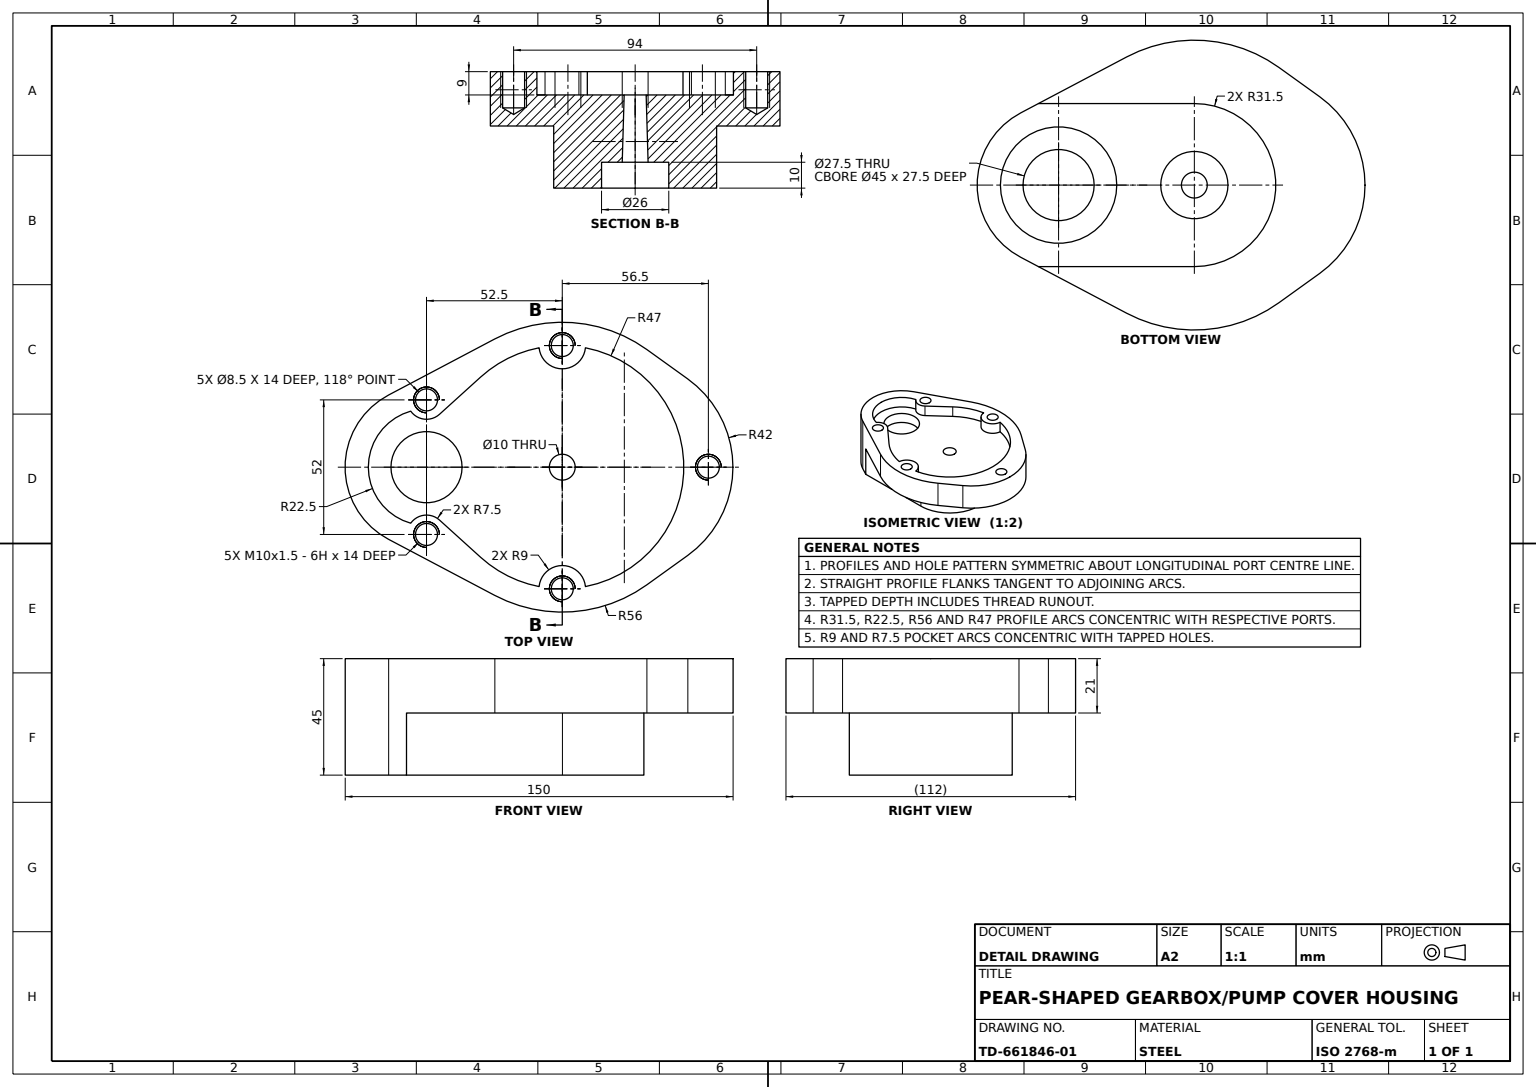
SolidWorks part; units mm, degrees
material "Plain Carbon Steel"
ref_plane "Front Plane" through (0, 0, 0) normal (0, 0, 1) x (1, 0, 0)
ref_plane "Top Plane" through (0, 0, 0) normal (0, 1, 0) x (1, 0, 0)
ref_plane "Right Plane" through (0, 0, 0) normal (1, 0, 0) x (0, 0, -1)
sketch "Flange Base Profile" plane through (0, 0, 0) normal (0, 1, 0) x (1, 0, 0)
  line L0 (-49.5283, 26.3667) -> (-27.8596, -14.7)
  line L1 (27.8596, -14.7) -> (49.5283, 26.3667)
  line L2 (0, 0) -> (0, 118.5) construction
  line L3 (-45.485, 85.1667) -> (-34.1138, 101)
  line L4 (45.485, 85.1667) -> (34.1138, 101)
  arc A0 (-27.8596, -14.7) -> (27.8596, -14.7) centre (0, 0) ccw
  arc A1 (49.5283, 26.3667) -> (45.485, 85.1667) centre (0, 52.5) ccw
  arc A2 (34.1138, 101) -> (-34.1138, 101) centre (0, 76.5) ccw
  arc A3 (-45.485, 85.1667) -> (-49.5283, 26.3667) centre (0, 52.5) ccw
  point P9 (0, -31.5)
  point P15 (0, 109)
  dimension "D1" = 31.5
  dimension "D2" = 56
  dimension "D4" = 42
  dimension "D3" = 52.5
  dimension "D5" = 150
  dimension "D6" = 56.5
extrude "Flange Base 21mm" add sketch "Flange Base Profile" along normal blind 21
sketch "Port Pocket Profile" plane through (0, 21, 0) normal (0, 1, 0) x (1, 0, 0)
  line L0 (0, 0) -> (0, -14.6458) construction
  line L1 (-21.5965, 6.3121) -> (-20.4378, 5.0311)
  line L2 (34.8564, 20.9717) -> (20.4378, 5.0311)
  line L3 (-34.8564, 20.9717) -> (-21.5965, 6.3121)
  arc A0 (-46.1383, 43.5413) -> (-34.8564, 20.9717) centre (0, 52.5) ccw
  arc A1 (49.5283, 26.3667) -> (45.485, 85.1667) centre (0, 52.5) ccw construction
  arc A2 (-46.1383, 43.5413) -> (-46.1383, 61.4587) centre (-47, 52.5) ccw
  arc A3 (-46.1383, 61.4587) -> (-46.1383, 43.5413) centre (-47, 52.5) ccw construction
  arc A4 (-46.1383, 61.4587) -> (-46.1383, 43.5413) centre (0, 52.5) ccw construction
  arc A5 (46.1383, 43.5413) -> (46.1383, 61.4587) centre (47, 52.5) cw
  arc A6 (46.1383, 43.5413) -> (46.1383, 61.4587) centre (0, 52.5) ccw construction
  arc A7 (46.1383, 61.4587) -> (-46.1383, 61.4587) centre (0, 52.5) ccw
  arc A8 (-21.5965, 6.3121) -> (-21.6538, 6.1124) centre (0, 0) ccw construction
  arc A9 (-20.1391, 10.0333) -> (20.1391, 10.0333) centre (0, 52.5) ccw construction
  arc A10 (34.8564, 20.9717) -> (46.1383, 43.5413) centre (0, 52.5) ccw
  arc A11 (20.1391, 10.0333) -> (-20.1391, 10.0333) centre (0, 0) ccw construction
  arc A12 (-21.6538, -6.1124) -> (-20.4378, 5.0311) centre (-26, 0) ccw
  arc A13 (21.6538, -6.1124) -> (20.4378, 5.0311) centre (26, 0) cw
  arc A14 (-20.1391, 10.0333) -> (-21.5965, 6.3121) centre (0, 0) ccw construction
  arc A15 (-34.8564, 20.9717) -> (-20.1391, 10.0333) centre (0, 52.5) ccw construction
  arc A16 (21.5965, 6.3121) -> (20.1391, 10.0333) centre (0, 0) ccw construction
  arc A17 (20.1391, 10.0333) -> (34.8564, 20.9717) centre (0, 52.5) ccw construction
  arc A18 (-21.6538, 6.1124) -> (-21.6538, -6.1124) centre (-26, 0) ccw construction
  arc A19 (-21.6538, 6.1124) -> (-21.6538, -6.1124) centre (0, 0) ccw construction
  arc A20 (-21.6538, -6.1124) -> (21.6538, -6.1124) centre (0, 0) ccw
  arc A21 (21.6538, -6.1124) -> (21.6538, 6.1124) centre (0, 0) ccw construction
  arc A22 (21.6538, 6.1124) -> (21.5965, 6.3121) centre (0, 0) ccw construction
  arc A23 (21.6538, 6.1124) -> (21.6538, -6.1124) centre (26, 0) cw construction
  arc A24 (-20.4378, 5.0311) -> (-21.6538, 6.1124) centre (-26, 0) ccw construction
  arc A25 (20.4378, 5.0311) -> (21.6538, 6.1124) centre (26, 0) cw construction
  dimension "D1" = 47
  dimension "D2" = 9
  dimension "D3" = 22.5
  dimension "D4" = 7.5
  dimension "D5" = 52
extrude "Port Pocket 9mm Deep" cut sketch "Port Pocket Profile" against normal blind 9
hole_wizard "Tapped Hole M10 Drill Ø8.5" positions "3DSketch2" profile "Sketch4" hole size "M10" standard "ISO"
sketch3d "3DSketch2"
  line L0 (-47, 12, -52.5) -> (-47, 21, -52.5) construction
  arc A0 (-46.1383, 21, -61.4587) -> (-46.1383, 21, -43.5413) centre (-47, 21, -52.5) ccw construction
  arc A1 (46.1383, 21, -43.5413) -> (46.1383, 21, -61.4587) centre (47, 21, -52.5) ccw construction
  arc A2 (21.6538, 21, 6.1124) -> (20.4378, 21, -5.0311) centre (26, 21, 0) ccw construction
  arc A3 (-20.4378, 21, -5.0311) -> (-21.6538, 21, 6.1124) centre (-26, 21, 0) ccw construction
  point P0 (0, 21, -109)
  point P5 (-47, 21, -52.5)
  point P9 (47, 21, -52.5)
  point P11 (-26, 21, 0)
  point P13 (26, 21, 0)
  point P18 (-47, 12, -52.5)
  point P22 (47, 12, -52.5)
  point P26 (26, 13.5, 0)
  point P30 (-26, 13.5, 0)
sketch "Sketch4" plane through (0, 21, -109) normal (1, 0, 0) x (0, 0, 1)
  line L0 (0, 0) -> (0, 16.5537)
  line L1 (0, 16.5537) -> (4.25, 14)
  line L2 (4.25, 14) -> (4.25, 0)
  line L5 (4.25, 0) -> (0, 0)
  line L10 (0, 16.5537) -> (-4.25, 14) construction
  line L11 (0, -6.35) -> (0, 107.95) construction
  dimension "Hole Dia." = 8.5
  dimension "Hole Depth" = 14
  dimension "Drill Angle" = 118
sketch "Port Boss Profile" plane through (0, 0, 0) normal (0, -1, 0) x (1, 0, 0)
  line L6 (0, 0) -> (0, -52.5) construction
  line L11 (31.5, 0) -> (31.5, -52.5)
  line L12 (-31.5, 0) -> (-31.5, -52.5)
  line L15 (-31.5, 0) -> (-31.5, 7.8008)
  line L17 (-49.5283, -26.3667) -> (-27.8596, 14.7) construction
  line L18 (-31.5, 7.8008) -> (-27.8596, 14.7)
  line L19 (31.5, 0) -> (31.5, 7.8008)
  line L20 (27.8596, 14.7) -> (49.5283, -26.3667) construction
  line L21 (27.8596, 14.7) -> (31.5, 7.8008)
  arc A3 (27.8596, 14.7) -> (-27.8596, 14.7) centre (0, 0) ccw
  arc A6 (-31.5, -52.5) -> (31.5, -52.5) centre (0, -52.5) ccw
  arc A7 (-27.8596, 14.7) -> (-31.5, 0) centre (0, 0) ccw construction
  arc A8 (31.5, 0) -> (27.8596, 14.7) centre (0, 0) ccw construction
  dimension "D1" = 52.5
  dimension "D2" = 31.5
extrude "Port Boss 24mm" add sketch "Port Boss Profile" along normal blind 24
hole_wizard "Main Port C-Bore Ø27.5" positions "3DSketch3" profile "Sketch7" legacy
sketch3d "3DSketch3"
  arc A0 (27.8596, -24, 14.7) -> (-27.8596, -24, 14.7) centre (0, -24, 0) ccw construction
  point P0 (0, 0, 0)
  point P3 (0, -24, 0)
  point P9 (0, -55.5, 0)
sketch "Sketch7" plane through (0, -24, 0) normal (1, 0, 0) x (0, 0, -1)
  line L0 (0, 0) -> (0, 99.6165)
  line L1 (0, 99.6165) -> (13.75, 99.6165)
  line L2 (13.75, 99.6165) -> (13.75, 27.5)
  line L3 (13.75, 27.5) -> (22.5, 27.5)
  line L4 (22.5, 27.5) -> (22.5, 0)
  line L5 (22.5, 0) -> (0, 0)
  line L6 (0, 110) -> (0, -10) construction
  dimension "Diameter" = 27.5
  dimension "Depth" = 100
  dimension "C-Bore Diameter" = 45
  dimension "C-Bore Depth" = 27.5
hole_wizard "Secondary Port C-Bore Ø10" positions "3DSketch4" profile "Sketch8" legacy
sketch3d "3DSketch4"
  arc A0 (-31.5, 0, -52.5) -> (31.5, 0, -52.5) centre (0, 0, -52.5) ccw construction
  point P0 (0, -24, -52.5)
  point P6 (0, -31.5, -52.5)
sketch "Sketch8" plane through (0, -24, -52.5) normal (1, 0, 0) x (0, 0, -1)
  line L0 (0, 0) -> (0, 99.6795)
  line L1 (0, 99.6795) -> (5, 99.6795)
  line L2 (5, 99.6795) -> (5, 10)
  line L3 (5, 10) -> (13, 10)
  line L4 (13, 10) -> (13, 0)
  line L5 (13, 0) -> (0, 0)
  line L6 (0, 110) -> (0, -10) construction
  dimension "Diameter" = 10
  dimension "Depth" = 100
  dimension "C-Bore Diameter" = 26
  dimension "C-Bore Depth" = 10
